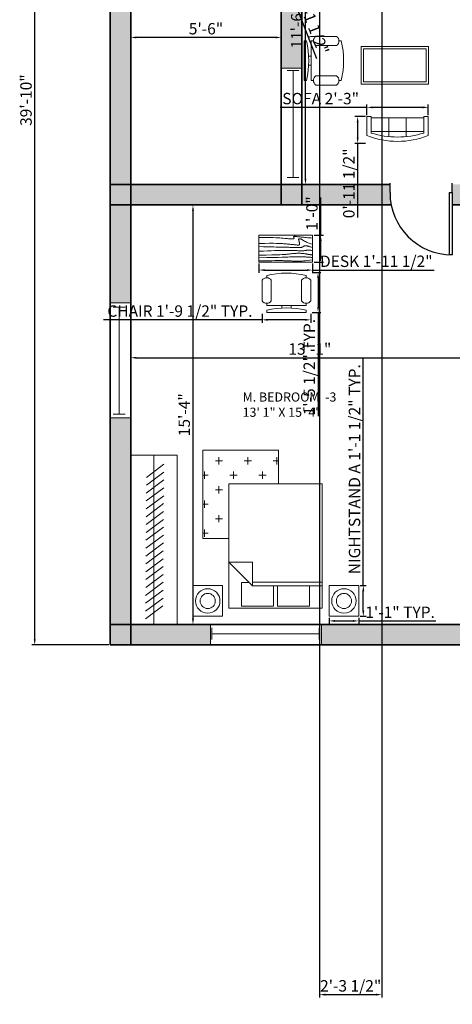
# Model space of a CAD drawing. Units: millimetres. Extents: x 2768 to 4359, y 795 to 1583.
# Tile 1 of 13: x 2772 to 2961, y 854 to 1286. Entities that reach past the tile are written whole.
import ezdxf

# ---------------------------------------------------------------- set-up
doc = ezdxf.new("R2010")
doc.units = ezdxf.units.MM
for name, color, linetype, lineweight in [('A-ANNO-DIMS', 90, 'Continuous', 18), ('A-AREA-IDEN', 190, 'Continuous', 18), ('A-FLOR-CASE', 50, 'Continuous', 18), ('A-FLOR-CASE-PATT', 50, 'Continuous', 13), ('A-FURN-PATT', 50, 'Continuous', 9), ('A-WALL-PATT', 140, 'Continuous', 9), ('doors', 10, 'Continuous', 25), ('furniture', 50, 'Continuous', 18), ('walls', 140, 'Continuous', 35), ('windows', 30, 'Continuous', 18)]:
    doc.layers.add(name, color=color, linetype=linetype, lineweight=lineweight)
doc.styles.get("Standard").update_dxf_attribs({"font": 'arial.ttf'})
doc.dimstyles.new('ISO-25', dxfattribs={"dimtxt": 5, "dimasz": 2.5, "dimexe": 1.25, "dimexo": 0.625, "dimtad": 1, "dimdec": 0, "dimlunit": 3, "dimtxsty": 'Standard', "dimcen": 2.5, "dimadec": 0, "dimazin": 0, "dimtfac": 1, "dimtdec": 0, "dimtmove": 0, "dimatfit": 3, "dimfxl": 1, "dimarcsym": 0})

# ---------------------------------------------------------------- blocks, each defined once
blk = doc.blocks.new('*U2')
for p, q in [((0, 0), (0, -6)), ((40, 0), (40, -6))]:
    blk.add_line(p, q)
blk.add_lwpolyline([(0, 0), (0, 40), (1.75, 40), (1.75, 0)], close=True)
blk.add_arc((0, 0), 40, 0, 90)
blk = doc.blocks.new('*U4')
for p, q in [((0, 4), (0, 0)), ((36, 4), (36, 0)), ((0, 2), (36, 2))]:
    blk.add_line(p, q)
blk = doc.blocks.new('Bed - Queen')
for p, q in [((0, -80.00003), (0, 0)), ((0, 0), (59.99999, 0)), ((59.99999, 0), (59.99999, -80.00003)), ((7.99999, -1.2), (28.79998, -1.2)), ((7.99999, -14.4), (7.99999, -1.2)), ((28.79998, -1.2), (28.79998, -14.4)), ((31.19999, -1.2), (51.99999, -1.2)), ((31.19999, -14.4), (31.19999, -1.2)), ((51.99999, -1.2), (51.99999, -16.4)), ((0, -14.4), (44.8, -14.4)), ((44.8, -16.8), (0, -16.8)), ((59.99999, -29.6), (44.8, -14.4)), ((44.8, -14.4), (44.8, -29.6)), ((51.99999, -16.4), (46.79936, -16.4)), ((44.8, -29.6), (59.99999, -29.6)), ((59.99999, -80.00003), (0, -80.00003))]:
    blk.add_line(p, q)
blk = doc.blocks.new('Chair - Desk')
for p, q in [((-8.5, 0), (-8.5, -1)), ((-8.5, 0), (8.5, 0)), ((8.5, 0), (8.5, -1)), ((-8.5, -3), (-8.5, -4)), ((-8.5, -3), (8.5, -3)), ((-2, -3), (-2, -1.9355)), ((2, -1.9576), (2, -3)), ((8.5, -3), (8.5, -4)), ((-10.5, -5), (-10.5, -14)), ((-6.5, -14), (-6.5, -5)), ((6.5, -5), (6.5, -14)), ((10.5, -14), (10.5, -5)), ((-8.5, -15), (-8.5, -16)), ((8.5, -15), (8.5, -16))]:
    blk.add_line(p, q)
for centre, radius, start, end in [((-8.5, -6.5), 2.5, 36.8699, 143.1301), ((0, 34.625), 36.625, 256.5803, 283.4197), ((8.5, -6.5), 2.5, 36.8699, 143.1301), ((-8.5, -12.5), 2.5, 216.8699, 323.1301), ((0, 19.625), 36.625, 256.5803, 283.4197), ((8.5, -12.5), 2.5, 216.8699, 323.1301)]:
    blk.add_arc(centre, radius, start, end)
blk = doc.blocks.new('Sofa - Roundback 7 ft.')
for p, q in [((-36.000027, -34), (-36.000027, -11.4696)), ((-35.999844, -13.3819), (35.9998, -13.3819)), ((-12.00002, -32.4421), (-12.00003, -6.5971)), ((11.99997, -32.4421), (11.99998, -6.5971)), ((35.99998, -34), (35.99998, -11.4696)), ((-36.000027, -32.4421), (35.99998, -32.4421))]:
    blk.add_line(p, q)
for points in [[(-36.000027, -34), (-42.000027, -34), (-42.000027, -8)], [(41.99998, -8), (41.99998, -34), (35.99998, -34)]]:
    blk.add_lwpolyline(points)
for centre, radius, start, end in [((0, -114.25), 114.25, 68.43141, 111.5686), ((-0.00001, -127.1968), 121.1968, 72.72033, 107.2797)]:
    blk.add_arc(centre, radius, start, end)
blk = doc.blocks.new('Table - Rectangular Woodgrain 60 x 30 in.')
for p, q in [((0, 0), (0, -30)), ((60, 0), (0, 0)), ((60, -30), (60, 0)), ((0, -30), (60, -30))]:
    blk.add_line(p, q)
for points in [[(0, -2.4), (4.8155, -2.418), (9.0302, -2.4688), (12.709, -2.5477), (15.9167, -2.65), (18.7181, -2.7711), (21.1781, -2.9063), (23.3616, -3.0508), (25.3333, -3.2), (27.1477, -3.3495), (28.8172, -3.4958), (30.3437, -3.636), (31.7291, -3.7667), (32.9756, -3.8849), (34.0849, -3.9875), (35.059, -4.0714), (35.9, -4.1334), (36.6114, -4.1711), (37.2041, -4.1854), (37.6906, -4.1779), (38.0833, -4.15), (38.3948, -4.1034), (38.6375, -4.0396), (38.8239, -3.9602), (38.9666, -3.8667), (39.0764, -3.7608), (39.1573, -3.6448), (39.2116, -3.521), (39.2416, -3.3917), (39.2498, -3.2593), (39.2385, -3.1261), (39.21, -2.9944), (39.1666, -2.8667), (39.111, -2.7447), (39.0468, -2.6281), (38.978, -2.5163), (38.9083, -2.4083), (38.8418, -2.3035), (38.7823, -2.201), (38.7337, -2.1001), (38.7, -2), (38.6844, -1.9003), (38.6875, -1.8021), (38.7094, -1.707), (38.75, -1.6167), (38.8094, -1.5326), (38.8875, -1.4563), (38.9844, -1.3893), (39.1, -1.3333), (39.2351, -1.2896), (39.3937, -1.2583), (39.5804, -1.2396), (39.8, -1.2333), (40.057, -1.2396), (40.3562, -1.2583), (40.7023, -1.2896), (41.1, -1.3333), (41.5547, -1.3895), (42.0755, -1.4573), (42.6721, -1.5361), (43.3542, -1.625), (44.1316, -1.7233), (45.014, -1.8302), (46.0114, -1.9449), (47.1333, -2.0667), (48.3862, -2.1947), (49.7625, -2.3281), (51.2513, -2.4663), (52.8416, -2.6083), (54.5226, -2.7535), (56.2833, -2.9011), (58.1127, -3.0501), (60, -3.2)], [(0, -9.2), (6.5759, -9.0858), (11.9385, -9.0365), (16.2527, -9.0418), (19.6833, -9.0917), (22.3952, -9.1759), (24.5531, -9.2844), (26.322, -9.4069), (27.8666, -9.5333), (29.3241, -9.6553), (30.7203, -9.7719), (32.0532, -9.8837), (33.3208, -9.9917), (34.5213, -10.0965), (35.6526, -10.199), (36.7128, -10.2999), (37.7, -10.4), (38.6129, -10.4996), (39.4531, -10.5969), (40.223, -10.6895), (40.925, -10.775), (41.5613, -10.8512), (42.1344, -10.9156), (42.6465, -10.966), (43.1, -11), (43.4976, -11.0158), (43.8437, -11.0136), (44.143, -10.9942), (44.4, -10.9583), (44.6195, -10.9069), (44.8062, -10.8406), (44.9648, -10.7603), (45.1, -10.6667), (45.2155, -10.5598), (45.3114, -10.4365), (45.3871, -10.2929), (45.4416, -10.125), (45.4743, -9.929), (45.4844, -9.7011), (45.4709, -9.4371), (45.4333, -9.1333), (45.3716, -8.7883), (45.2896, -8.4104), (45.1919, -8.0107), (45.0833, -7.6), (44.9685, -7.1893), (44.8521, -6.7896), (44.7388, -6.4117), (44.6333, -6.0667), (44.54, -5.7628), (44.4614, -5.4979), (44.4001, -5.2675), (44.3583, -5.0667), (44.3384, -4.8909), (44.3427, -4.7354), (44.3736, -4.5956), (44.4333, -4.4667), (44.5236, -4.3453), (44.6427, -4.2333), (44.7884, -4.1339), (44.9583, -4.05), (45.1501, -3.9849), (45.3614, -3.9417), (45.59, -3.9234), (45.8333, -3.9333), (46.0915, -3.9749), (46.3734, -4.0531), (46.6906, -4.1736), (47.0542, -4.3417), (47.4756, -4.5629), (47.9661, -4.8427), (48.5372, -5.1866), (49.2, -5.6), (49.9676, -6.0844), (50.8594, -6.625), (51.8965, -7.2031), (53.1, -7.8), (54.491, -8.3969), (56.0906, -8.975), (57.9199, -9.5156), (60, -10)], [(0, -12.8), (5.1847, -12.9322), (9.6213, -13.0323), (13.3963, -13.1059), (16.5958, -13.1583), (19.3063, -13.1952), (21.614, -13.2219), (23.6054, -13.2439), (25.3666, -13.2667), (26.9728, -13.2947), (28.4531, -13.3281), (29.8256, -13.3663), (31.1083, -13.4083), (32.3191, -13.4535), (33.476, -13.501), (34.597, -13.5501), (35.7, -13.6), (36.7984, -13.6497), (37.8875, -13.6979), (38.9578, -13.743), (40, -13.7833), (41.0047, -13.8174), (41.9625, -13.8438), (42.864, -13.8607), (43.7, -13.8667), (44.4631, -13.8604), (45.1552, -13.8417), (45.7801, -13.8104), (46.3416, -13.7667), (46.8439, -13.7104), (47.2906, -13.6417), (47.6858, -13.5604), (48.0333, -13.4667), (48.3375, -13.3608), (48.6042, -13.2448), (48.8396, -13.121), (49.05, -12.9917), (49.2417, -12.8593), (49.4208, -12.7261), (49.5937, -12.5944), (49.7667, -12.4667), (49.9452, -12.3451), (50.1323, -12.2313), (50.3303, -12.1268), (50.5416, -12.0333), (50.7686, -11.9524), (51.0135, -11.8854), (51.2788, -11.8341), (51.5666, -11.8), (51.8785, -11.7843), (52.2116, -11.7865), (52.562, -11.8059), (52.926, -11.8417), (53.2998, -11.8931), (53.6795, -11.9594), (54.0614, -12.0397), (54.4416, -12.1333), (54.8223, -12.2401), (55.2293, -12.3625), (55.6942, -12.5037), (56.2489, -12.6667), (56.9251, -12.8547), (57.7545, -13.0708), (58.7689, -13.3182), (60, -13.6)], [(0, -18), (5.124, -17.7273), (9.6609, -17.5057), (13.6705, -17.3303), (17.2125, -17.1958), (20.3467, -17.0973), (23.1328, -17.0297), (25.6307, -16.9878), (27.9, -16.9667), (29.9928, -16.9617), (31.9302, -16.9703), (33.7254, -16.9907), (35.3917, -17.0208), (36.9423, -17.0588), (38.3906, -17.1026), (39.7499, -17.1503), (41.0333, -17.2), (42.2519, -17.2496), (43.4073, -17.2969), (44.4986, -17.3395), (45.525, -17.375), (46.4858, -17.4012), (47.3802, -17.4156), (48.2074, -17.416), (48.9667, -17.4), (49.6583, -17.3662), (50.2872, -17.3167), (50.8595, -17.2547), (51.3812, -17.1833), (51.8584, -17.1057), (52.2971, -17.025), (52.7034, -16.9443), (53.0833, -16.8667), (53.443, -16.7951), (53.789, -16.7313), (54.128, -16.6768), (54.4666, -16.6334), (54.8115, -16.6024), (55.1693, -16.5854), (55.5465, -16.5841), (55.95, -16.6), (56.3828, -16.6337), (56.8346, -16.6823), (57.2915, -16.7418), (57.7396, -16.8084), (58.165, -16.878), (58.5539, -16.9469), (58.8924, -17.0111), (59.1666, -17.0667), (59.3679, -17.1107), (59.5078, -17.1438), (59.6032, -17.1675), (59.6708, -17.1833), (59.7275, -17.193), (59.7901, -17.1979), (59.8753, -17.1998), (60, -17.2)], [(0, -22.4), (8.0098, -22.2501), (14.4094, -22.1011), (19.4168, -21.9535), (23.25, -21.8083), (26.1269, -21.6663), (28.2656, -21.5281), (29.884, -21.3947), (31.2, -21.2667), (32.3967, -21.1448), (33.5172, -21.0292), (34.5697, -20.9198), (35.5625, -20.8167), (36.5037, -20.7198), (37.4015, -20.6292), (38.2642, -20.5448), (39.1, -20.4667), (39.9164, -20.3951), (40.7187, -20.3313), (41.5117, -20.2768), (42.3, -20.2333), (43.0883, -20.2024), (43.8812, -20.1854), (44.6836, -20.1841), (45.5, -20.2), (46.3328, -20.234), (47.1747, -20.2844), (48.0163, -20.3488), (48.8479, -20.425), (49.66, -20.5106), (50.4429, -20.6031), (51.1872, -20.7004), (51.8833, -20.8), (52.5246, -20.8999), (53.1166, -20.9995), (53.6681, -21.0983), (54.1875, -21.1958), (54.6834, -21.2919), (55.1646, -21.3859), (55.6394, -21.4777), (56.1167, -21.5667), (56.6028, -21.6515), (57.0961, -21.7266), (57.5929, -21.7852), (58.0896, -21.8208), (58.5823, -21.8268), (59.0674, -21.7964), (59.5412, -21.723), (60, -21.6)], [(0, -25.2), (8.6355, -25.0504), (15.7026, -24.9031), (21.4049, -24.7606), (25.9458, -24.625), (29.529, -24.4988), (32.3578, -24.3844), (34.6359, -24.284), (36.5667, -24.2), (38.3213, -24.1341), (39.9417, -24.0854), (41.437, -24.0523), (42.8167, -24.0333), (44.0901, -24.0268), (45.2667, -24.0313), (46.3557, -24.0451), (47.3667, -24.0667), (48.309, -24.0947), (49.1928, -24.1287), (50.0284, -24.168), (50.826, -24.2125), (51.5959, -24.2617), (52.3483, -24.3151), (53.0935, -24.3725), (53.8417, -24.4334), (54.6009, -24.497), (55.3699, -24.561), (56.1454, -24.6226), (56.9239, -24.6792), (57.7021, -24.7279), (58.4764, -24.7662), (59.2435, -24.7911), (60, -24.8)], [(0, -28.8), (5.6867, -28.6681), (10.45, -28.5698), (14.407, -28.5012), (17.675, -28.4584), (20.3711, -28.4374), (22.6125, -28.4344), (24.5164, -28.4455), (26.2, -28.4667), (27.762, -28.4947), (29.2276, -28.5281), (30.6033, -28.5663), (31.8958, -28.6084), (33.1118, -28.6535), (34.2578, -28.7011), (35.3405, -28.7501), (36.3666, -28.8), (37.3443, -28.8497), (38.288, -28.8974), (39.2137, -28.9412), (40.1375, -28.9792), (41.0753, -29.0093), (42.0432, -29.0297), (43.0572, -29.0384), (44.1333, -29.0333), (45.2936, -29.0114), (46.5843, -28.9641), (48.0579, -28.8816), (49.7666, -28.7542), (51.7629, -28.5721), (54.0989, -28.3255), (56.8272, -28.0048), (60, -27.6)]]:
    blk.add_lwpolyline(points)
blk = doc.blocks.new('*D21')
at = {"layer": 'A-ANNO-DIMS', "color": 0, "lineweight": -2, "transparency": 16777216}
for p, q in [((2820.41, 1281.78), (2820.41, 1276.66)), ((2886.41, 1281.78), (2886.41, 1276.66)), ((2883.91, 1277.91), (2822.91, 1277.91))]:
    blk.add_line(p, q, dxfattribs=at)
at = {"layer": 'A-ANNO-DIMS', "color": 0, "transparency": 16777216}
for points in [[(2822.91, 1278.32), (2822.91, 1277.49), (2820.41, 1277.91)], [(2883.91, 1278.32), (2883.91, 1277.49), (2886.41, 1277.91)]]:
    blk.add_solid(points, dxfattribs=at)
at = {"layer": 'Defpoints', "color": 0, "transparency": 16777216}
for p in [(2820.41, 1282.41), (2886.41, 1282.41), (2820.41, 1277.91)]:
    blk.add_point(p, dxfattribs=at)
at = {"layer": 'A-ANNO-DIMS', "color": 0, "transparency": 16777216, "insert": (2853.41, 1281.08), "char_height": 5, "attachment_point": 5}
blk.add_mtext('5\'-6"', dxfattribs=at)
blk = doc.blocks.new('*D22')
at = {"layer": 'A-ANNO-DIMS', "color": 0, "lineweight": -2, "transparency": 16777216}
for p, q in [((2820.41, 1131.43), (2820.41, 1138.66)), ((2822.91, 1137.41), (2974.91, 1137.41)), ((2977.41, 1138.03), (2977.41, 1138.66))]:
    blk.add_line(p, q, dxfattribs=at)
at = {"layer": 'A-ANNO-DIMS', "color": 0, "transparency": 16777216}
for points in [[(2822.91, 1137.82), (2822.91, 1136.99), (2820.41, 1137.41)], [(2974.91, 1137.82), (2974.91, 1136.99), (2977.41, 1137.41)]]:
    blk.add_solid(points, dxfattribs=at)
at = {"layer": 'Defpoints', "color": 0, "transparency": 16777216}
for p in [(2977.41, 1137.41), (2977.41, 1137.41), (2820.41, 1130.8)]:
    blk.add_point(p, dxfattribs=at)
at = {"layer": 'A-ANNO-DIMS', "color": 0, "transparency": 16777216, "insert": (2898.91, 1140.59), "char_height": 5, "attachment_point": 5}
blk.add_mtext('13\'-1"', dxfattribs=at)
blk = doc.blocks.new('*D23')
at = {"layer": 'A-ANNO-DIMS', "color": 0, "lineweight": -2, "transparency": 16777216}
for p, q in [((2844.38, 1204.41), (2848.95, 1204.41)), ((2847.7, 1201.91), (2847.7, 1022.91)), ((2847.38, 1020.41), (2848.95, 1020.41))]:
    blk.add_line(p, q, dxfattribs=at)
at = {"layer": 'A-ANNO-DIMS', "color": 0, "transparency": 16777216}
for points in [[(2847.29, 1201.91), (2848.12, 1201.91), (2847.7, 1204.41)], [(2847.29, 1022.91), (2848.12, 1022.91), (2847.7, 1020.41)]]:
    blk.add_solid(points, dxfattribs=at)
at = {"layer": 'Defpoints', "color": 0, "transparency": 16777216}
for p in [(2843.76, 1204.41), (2846.76, 1020.41), (2847.7, 1020.41)]:
    blk.add_point(p, dxfattribs=at)
at = {"layer": 'A-ANNO-DIMS', "color": 0, "transparency": 16777216, "insert": (2844.52, 1112.41), "char_height": 5, "attachment_point": 5, "rotation": 90}
blk.add_mtext('15\'-4"', dxfattribs=at)
blk = doc.blocks.new('*D31')
at = {"layer": 'A-ANNO-DIMS', "color": 0, "lineweight": -2, "transparency": 16777216}
for p, q in [((2897.01, 1215.91), (2897.01, 1348.91)), ((2897.64, 1351.41), (2898.26, 1351.41)), ((2897.72, 1213.41), (2895.76, 1213.41))]:
    blk.add_line(p, q, dxfattribs=at)
at = {"layer": 'A-ANNO-DIMS', "color": 0, "transparency": 16777216}
for points in [[(2896.59, 1348.91), (2897.43, 1348.91), (2897.01, 1351.41)], [(2896.59, 1215.91), (2897.43, 1215.91), (2897.01, 1213.41)]]:
    blk.add_solid(points, dxfattribs=at)
at = {"layer": 'Defpoints', "color": 0, "transparency": 16777216}
for p in [(2897.01, 1351.41), (2897.01, 1351.41), (2898.34, 1213.41)]:
    blk.add_point(p, dxfattribs=at)
at = {"layer": 'A-ANNO-DIMS', "color": 0, "transparency": 16777216, "insert": (2893.83, 1282.41), "char_height": 5, "attachment_point": 5, "rotation": 90}
blk.add_mtext('11\'-6"', dxfattribs=at)
blk = doc.blocks.new('NIGHTSTAND-RECT-A')
blk.add_lwpolyline([(0, 13.48), (12.92, 13.48), (12.92, 0), (0, 0)], close=True)
for radius in [5.37, 3.33]:
    blk.add_circle((6.46, 6.74), radius)
blk = doc.blocks.new('*D83')
at = {"layer": 'A-ANNO-DIMS', "color": 0, "lineweight": -2, "transparency": 16777216}
for p, q in [((2870.86, 1339.78), (2874.98, 1341.38)), ((2874.71, 1338.6), (2882.05, 1319.7)), ((2880, 1316.23), (2884.12, 1317.83)), ((2882.95, 1317.37), (2901.88, 1268.61))]:
    blk.add_line(p, q, dxfattribs=at)
at = {"layer": 'A-ANNO-DIMS', "color": 0, "transparency": 16777216}
for points in [[(2875.1, 1338.75), (2874.33, 1338.45), (2873.81, 1340.93)], [(2882.44, 1319.85), (2881.66, 1319.55), (2882.95, 1317.37)]]:
    blk.add_solid(points, dxfattribs=at)
at = {"layer": 'Defpoints', "color": 0, "transparency": 16777216}
for p in [(2870.28, 1339.56), (2882.95, 1317.37), (2879.42, 1316)]:
    blk.add_point(p, dxfattribs=at)
at = {"layer": 'A-ANNO-DIMS', "color": 0, "transparency": 16777216, "insert": (2895.86, 1292.99), "char_height": 5, "attachment_point": 5, "rotation": 291.2165}
blk.add_mtext('CHAIR 2\'-1 1/2"', dxfattribs=at)
blk = doc.blocks.new('*D85')
at = {"layer": 'A-ANNO-DIMS', "color": 0, "lineweight": -2, "transparency": 16777216}
for p, q in [((2877.97, 1154.03), (2808.48, 1154.03)), ((2877.97, 1156.61), (2877.97, 1152.78)), ((2896.83, 1154.03), (2880.47, 1154.03)), ((2899.33, 1156.61), (2899.33, 1152.78))]:
    blk.add_line(p, q, dxfattribs=at)
at = {"layer": 'A-ANNO-DIMS', "color": 0, "transparency": 16777216}
for points in [[(2880.47, 1154.45), (2880.47, 1153.62), (2877.97, 1154.03)], [(2896.83, 1154.45), (2896.83, 1153.62), (2899.33, 1154.03)]]:
    blk.add_solid(points, dxfattribs=at)
at = {"layer": 'Defpoints', "color": 0, "transparency": 16777216}
for p in [(2877.97, 1157.23), (2877.97, 1154.03), (2899.33, 1157.23)]:
    blk.add_point(p, dxfattribs=at)
at = {"layer": 'A-ANNO-DIMS', "color": 0, "transparency": 16777216, "insert": (2841.98, 1157.24), "char_height": 5, "attachment_point": 5}
blk.add_mtext('CHAIR 1\'-9 1/2" TYP.', dxfattribs=at)
blk = doc.blocks.new('*D86')
at = {"layer": 'A-ANNO-DIMS', "color": 0, "lineweight": -2, "transparency": 16777216}
for p, q in [((2899.95, 1174.86), (2903.78, 1174.86)), ((2902.53, 1172.36), (2902.53, 1159.73)), ((2899.95, 1157.23), (2903.78, 1157.23)), ((2902.53, 1157.23), (2902.53, 1111.83))]:
    blk.add_line(p, q, dxfattribs=at)
at = {"layer": 'A-ANNO-DIMS', "color": 0, "transparency": 16777216}
for points in [[(2902.11, 1172.36), (2902.95, 1172.36), (2902.53, 1174.86)], [(2902.11, 1159.73), (2902.95, 1159.73), (2902.53, 1157.23)]]:
    blk.add_solid(points, dxfattribs=at)
at = {"layer": 'Defpoints', "color": 0, "transparency": 16777216}
for p in [(2899.33, 1174.86), (2899.33, 1157.23), (2902.53, 1157.23)]:
    blk.add_point(p, dxfattribs=at)
at = {"layer": 'A-ANNO-DIMS', "color": 0, "transparency": 16777216, "insert": (2899.32, 1133.28), "char_height": 5, "attachment_point": 5, "rotation": 90}
blk.add_mtext('1\'-5 1/2" TYP.', dxfattribs=at)
blk = doc.blocks.new('*D101')
at = {"layer": 'A-ANNO-DIMS', "color": 0, "lineweight": -2, "transparency": 16777216}
for p, q in [((2923.9, 1243.81), (2923.9, 1248.47)), ((2950.8, 1243.81), (2950.8, 1248.47)), ((2923.9, 1247.22), (2885.92, 1247.22)), ((2948.3, 1247.22), (2926.4, 1247.22))]:
    blk.add_line(p, q, dxfattribs=at)
at = {"layer": 'A-ANNO-DIMS', "color": 0, "transparency": 16777216}
for points in [[(2926.4, 1247.64), (2926.4, 1246.81), (2923.9, 1247.22)], [(2948.3, 1247.64), (2948.3, 1246.81), (2950.8, 1247.22)]]:
    blk.add_solid(points, dxfattribs=at)
at = {"layer": 'Defpoints', "color": 0, "transparency": 16777216}
for p in [(2923.9, 1247.22), (2923.9, 1243.19), (2950.8, 1243.19)]:
    blk.add_point(p, dxfattribs=at)
at = {"layer": 'A-ANNO-DIMS', "color": 0, "transparency": 16777216, "insert": (2903.66, 1250.44), "char_height": 5, "attachment_point": 5}
blk.add_mtext('SOFA 2\'-3"', dxfattribs=at)
blk = doc.blocks.new('*D102')
at = {"layer": 'A-ANNO-DIMS', "color": 0, "lineweight": -2, "transparency": 16777216}
for p, q in [((2923.28, 1243.19), (2918.62, 1243.19)), ((2919.87, 1240.69), (2919.87, 1233.95)), ((2923.28, 1231.45), (2918.62, 1231.45)), ((2919.87, 1231.45), (2919.87, 1198.87))]:
    blk.add_line(p, q, dxfattribs=at)
at = {"layer": 'A-ANNO-DIMS', "color": 0, "transparency": 16777216}
for points in [[(2919.45, 1240.69), (2920.28, 1240.69), (2919.87, 1243.19)], [(2919.45, 1233.95), (2920.28, 1233.95), (2919.87, 1231.45)]]:
    blk.add_solid(points, dxfattribs=at)
at = {"layer": 'Defpoints', "color": 0, "transparency": 16777216}
for p in [(2923.9, 1243.19), (2919.87, 1231.45), (2923.9, 1231.45)]:
    blk.add_point(p, dxfattribs=at)
at = {"layer": 'A-ANNO-DIMS', "color": 0, "transparency": 16777216, "insert": (2916.66, 1213.91), "char_height": 5, "attachment_point": 5, "rotation": 90}
blk.add_mtext('0\'-11 1/2"', dxfattribs=at)
blk = doc.blocks.new('*D113')
at = {"layer": 'A-ANNO-DIMS', "color": 0, "lineweight": -2, "transparency": 16777216}
for p, q in [((2876.62, 1178.77), (2876.62, 1174.61)), ((2879.12, 1175.86), (2897.64, 1175.86)), ((2900.14, 1178.77), (2900.14, 1174.61)), ((2900.14, 1175.86), (2953.43, 1175.86))]:
    blk.add_line(p, q, dxfattribs=at)
at = {"layer": 'A-ANNO-DIMS', "color": 0, "transparency": 16777216}
for points in [[(2879.12, 1176.28), (2879.12, 1175.45), (2876.62, 1175.86)], [(2897.64, 1176.28), (2897.64, 1175.45), (2900.14, 1175.86)]]:
    blk.add_solid(points, dxfattribs=at)
at = {"layer": 'Defpoints', "color": 0, "transparency": 16777216}
for p in [(2876.62, 1179.39), (2900.14, 1179.39), (2900.14, 1175.86)]:
    blk.add_point(p, dxfattribs=at)
at = {"layer": 'A-ANNO-DIMS', "color": 0, "transparency": 16777216, "insert": (2928.04, 1179.07), "char_height": 5, "attachment_point": 5}
blk.add_mtext('DESK 1\'-11 1/2"', dxfattribs=at)
blk = doc.blocks.new('*D114')
at = {"layer": 'A-ANNO-DIMS', "color": 0, "lineweight": -2, "transparency": 16777216}
for p, q in [((2903.67, 1191.15), (2903.67, 1207.72)), ((2900.77, 1191.15), (2904.92, 1191.15)), ((2903.67, 1181.89), (2903.67, 1188.65)), ((2900.77, 1179.39), (2904.92, 1179.39))]:
    blk.add_line(p, q, dxfattribs=at)
at = {"layer": 'A-ANNO-DIMS', "color": 0, "transparency": 16777216}
for points in [[(2903.25, 1188.65), (2904.09, 1188.65), (2903.67, 1191.15)], [(2903.25, 1181.89), (2904.09, 1181.89), (2903.67, 1179.39)]]:
    blk.add_solid(points, dxfattribs=at)
at = {"layer": 'Defpoints', "color": 0, "transparency": 16777216}
for p in [(2900.14, 1191.15), (2903.67, 1191.15), (2900.14, 1179.39)]:
    blk.add_point(p, dxfattribs=at)
at = {"layer": 'A-ANNO-DIMS', "color": 0, "transparency": 16777216, "insert": (2900.49, 1200.69), "char_height": 5, "attachment_point": 5, "rotation": 90}
blk.add_mtext('1\'-0"', dxfattribs=at)
blk = doc.blocks.new('*D117')
at = {"layer": 'A-ANNO-DIMS', "color": 0, "lineweight": -2, "transparency": 16777216}
for p, q in [((2922.35, 1037.47), (2922.35, 1137.05)), ((2920.95, 1037.47), (2923.6, 1037.47)), ((2922.35, 1026.48), (2922.35, 1034.97)), ((2920.95, 1023.98), (2923.6, 1023.98))]:
    blk.add_line(p, q, dxfattribs=at)
at = {"layer": 'A-ANNO-DIMS', "color": 0, "transparency": 16777216}
for points in [[(2921.93, 1034.97), (2922.77, 1034.97), (2922.35, 1037.47)], [(2921.93, 1026.48), (2922.77, 1026.48), (2922.35, 1023.98)]]:
    blk.add_solid(points, dxfattribs=at)
at = {"layer": 'Defpoints', "color": 0, "transparency": 16777216}
for p in [(2920.33, 1037.47), (2922.35, 1037.47), (2920.33, 1023.98)]:
    blk.add_point(p, dxfattribs=at)
at = {"layer": 'A-ANNO-DIMS', "color": 0, "transparency": 16777216, "insert": (2919.14, 1088.51), "char_height": 5, "attachment_point": 5, "rotation": 90}
blk.add_mtext('NIGHTSTAND A 1\'-1 1/2" TYP.', dxfattribs=at)
blk = doc.blocks.new('*D118')
at = {"layer": 'A-ANNO-DIMS', "color": 0, "lineweight": -2, "transparency": 16777216}
for p, q in [((2907.41, 1023.36), (2907.41, 1020.71)), ((2909.91, 1021.96), (2917.83, 1021.96)), ((2920.33, 1023.36), (2920.33, 1020.71)), ((2920.33, 1021.96), (2954.08, 1021.96))]:
    blk.add_line(p, q, dxfattribs=at)
at = {"layer": 'A-ANNO-DIMS', "color": 0, "transparency": 16777216}
for points in [[(2909.91, 1022.38), (2909.91, 1021.54), (2907.41, 1021.96)], [(2917.83, 1022.38), (2917.83, 1021.54), (2920.33, 1021.96)]]:
    blk.add_solid(points, dxfattribs=at)
at = {"layer": 'Defpoints', "color": 0, "transparency": 16777216}
for p in [(2907.41, 1023.98), (2920.33, 1023.98), (2920.33, 1021.96)]:
    blk.add_point(p, dxfattribs=at)
at = {"layer": 'A-ANNO-DIMS', "color": 0, "transparency": 16777216, "insert": (2938.46, 1025.1), "char_height": 5, "attachment_point": 5}
blk.add_mtext('1\'-1" TYP.', dxfattribs=at)
blk = doc.blocks.new('*D127')
at = {"layer": 'A-ANNO-DIMS', "color": 0, "lineweight": -2, "transparency": 16777216}
for p, q in [((2810.78, 1489.41), (2777.11, 1489.41)), ((2778.36, 1013.91), (2778.36, 1486.91)), ((2810.78, 1011.41), (2777.11, 1011.41))]:
    blk.add_line(p, q, dxfattribs=at)
at = {"layer": 'A-ANNO-DIMS', "color": 0, "transparency": 16777216}
for points in [[(2777.94, 1486.91), (2778.77, 1486.91), (2778.36, 1489.41)], [(2777.94, 1013.91), (2778.77, 1013.91), (2778.36, 1011.41)]]:
    blk.add_solid(points, dxfattribs=at)
at = {"layer": 'Defpoints', "color": 0, "transparency": 16777216}
for p in [(2778.36, 1489.41), (2811.41, 1489.41), (2811.41, 1011.41)]:
    blk.add_point(p, dxfattribs=at)
at = {"layer": 'A-ANNO-DIMS', "color": 0, "transparency": 16777216, "insert": (2775.18, 1250.41), "char_height": 5, "attachment_point": 5, "rotation": 90}
blk.add_mtext('39\'-10"', dxfattribs=at)
blk = doc.blocks.new('*D133')
at = {"layer": 'A-ANNO-DIMS', "color": 0, "lineweight": -2, "transparency": 16777216}
for p, q in [((2903.16, 1350.78), (2903.16, 856.79)), ((2930.46, 1350.78), (2930.46, 856.79)), ((2905.66, 858.04), (2927.96, 858.04))]:
    blk.add_line(p, q, dxfattribs=at)
at = {"layer": 'A-ANNO-DIMS', "color": 0, "transparency": 16777216}
for points in [[(2905.66, 858.46), (2905.66, 857.63), (2903.16, 858.04)], [(2927.96, 858.46), (2927.96, 857.63), (2930.46, 858.04)]]:
    blk.add_solid(points, dxfattribs=at)
at = {"layer": 'Defpoints', "color": 0, "transparency": 16777216}
for p in [(2903.16, 1351.41), (2930.46, 1351.41), (2930.46, 858.04)]:
    blk.add_point(p, dxfattribs=at)
at = {"layer": 'A-ANNO-DIMS', "color": 0, "transparency": 16777216, "insert": (2916.81, 861.25), "char_height": 5, "attachment_point": 5}
blk.add_mtext('2\'-3 1/2"', dxfattribs=at)

msp = doc.modelspace()

# ---------------------------------------------------------------- hatches: boundary and pattern name
at = {"layer": 'A-FLOR-CASE-PATT'}
h = msp.add_hatch(dxfattribs=at)
h.set_pattern_fill('ANSI31', color=256, scale=0.865728, angle=-8.151, style=0)
h.paths.add_polyline_path([(2834.54, 1027.06), (2826.88, 1021.32), (2827.3, 1086.9), (2834.96, 1092.64)])
at = {"layer": 'A-FURN-PATT'}
h = msp.add_hatch(dxfattribs=at)
h.set_pattern_fill('CROSS', color=256)
h.paths.add_polyline_path([(2885.16, 1096.89), (2852.08, 1096.89), (2852.08, 1058.14), (2863.47, 1058.14), (2863.47, 1082.02), (2885.16, 1082.02)])
at = {"layer": 'A-WALL-PATT'}
h = msp.add_hatch(color=256, dxfattribs=at)
h.dxf.hatch_style = 1
h.paths.add_polyline_path([(2820.41, 1480.41), (2811.41, 1480.41), (2811.41, 1360.41), (2820.41, 1360.41)])
h.paths.add_polyline_path([(2820.41, 1489.41), (2811.41, 1489.41), (2811.41, 1480.41), (2820.41, 1480.41)])
h.paths.add_polyline_path([(2845.83, 1489.41), (2820.41, 1489.41), (2820.41, 1480.41), (2845.83, 1480.41)])
h.paths.add_polyline_path([(2940.41, 1489.41), (2894.95, 1489.41), (2894.95, 1480.41), (2940.41, 1480.41)])
h.paths.add_polyline_path([(2949.41, 1489.41), (2940.41, 1489.41), (2940.41, 1480.41), (2949.41, 1480.41)])
h.paths.add_polyline_path([(2949.41, 1480.41), (2940.41, 1480.41), (2940.41, 1433.68), (2943.15, 1433.68), (2949.41, 1433.68)])
h.paths.add_polyline_path([(2964.2, 1489.41), (2949.41, 1489.41), (2949.41, 1480.41), (2964.2, 1480.41)])
h.paths.add_polyline_path([(3018.41, 1489.41), (3009.41, 1489.41), (3009.41, 1480.41), (3018.41, 1480.41)])
h.paths.add_polyline_path([(3009.41, 1489.41), (2990.92, 1489.41), (2990.92, 1480.41), (3009.41, 1480.41)])
h.paths.add_polyline_path([(3018.41, 1480.41), (3009.41, 1480.41), (3009.41, 1384.41), (3018.41, 1384.41)])
h.paths.add_polyline_path([(3009.41, 1384.41), (2949.41, 1384.41), (2949.41, 1375.41), (3009.41, 1375.41)])
h.paths.add_polyline_path([(3018.41, 1384.41), (3009.41, 1384.41), (3009.41, 1375.41), (3018.41, 1375.41)])
h.paths.add_polyline_path([(2949.41, 1384.41), (2940.41, 1384.41), (2940.41, 1375.41), (2949.41, 1375.41)])
h.paths.add_polyline_path([(2949.41, 1413.64, -0.075856), (2943.15, 1412.69), (2940.41, 1412.69), (2940.41, 1384.41), (2949.41, 1384.41)])
h.paths.add_polyline_path([(2949.41, 1375.41), (2940.41, 1375.41), (2940.41, 1360.41), (2949.41, 1360.41)])
h.paths.add_polyline_path([(2949.41, 1360.41), (2940.41, 1360.41), (2940.41, 1351.41), (2949.41, 1351.41)])
h.paths.add_polyline_path([(2940.41, 1360.41), (2929.82, 1360.41, -0.054277), (2930.46, 1354.53), (2930.46, 1351.41), (2940.41, 1351.41)])
h.paths.add_polyline_path([(2903.16, 1354.53), (2903.16, 1360.41), (2895.41, 1360.41), (2895.41, 1351.41), (2903.16, 1351.41)])
h.paths.add_polyline_path([(2886.41, 1360.41), (2820.41, 1360.41), (2820.41, 1351.41), (2886.41, 1351.41)])
h.paths.add_polyline_path([(2895.41, 1360.41), (2886.41, 1360.41), (2886.41, 1351.41), (2895.41, 1351.41)])
h.paths.add_polyline_path([(2820.41, 1360.41), (2811.41, 1360.41), (2811.41, 1351.41), (2820.41, 1351.41)])
h.paths.add_polyline_path([(2820.41, 1351.41), (2811.41, 1351.41), (2811.41, 1213.41), (2820.41, 1213.41)])
h.paths.add_polyline_path([(2886.41, 1213.41), (2820.41, 1213.41), (2820.41, 1204.41), (2886.41, 1204.41)])
h.paths.add_polyline_path([(2820.41, 1213.41), (2811.41, 1213.41), (2811.41, 1204.41), (2820.41, 1204.41)])
h.paths.add_polyline_path([(2895.41, 1302), (2886.41, 1302), (2886.41, 1264.47), (2895.41, 1264.47)])
h.paths.add_polyline_path([(2934.05, 1209.82), (2934.05, 1213.41), (2895.41, 1213.41), (2895.41, 1204.41), (2934.59, 1204.41, -0.049949)])
h.paths.add_polyline_path([(2895.41, 1213.41), (2886.41, 1213.41), (2886.41, 1204.41), (2895.41, 1204.41)])
h.paths.add_polyline_path([(3078.41, 1384.41), (3018.41, 1384.41), (3018.41, 1375.41), (3078.41, 1375.41)])
h.paths.add_polyline_path([(3087.41, 1433.68), (3084.62, 1433.68), (3078.41, 1433.68), (3078.41, 1384.41), (3087.41, 1384.41)])
h.paths.add_polyline_path([(3087.41, 1384.41), (3078.41, 1384.41), (3078.41, 1375.41), (3087.41, 1375.41)])
h.paths.add_polyline_path([(3087.41, 1375.41), (3078.41, 1375.41), (3078.41, 1360.41), (3087.41, 1360.41)])
h.paths.add_polyline_path([(3087.41, 1360.41), (3078.41, 1360.41), (3078.41, 1351.41), (3087.41, 1351.41)])
h.paths.add_polyline_path([(3093.5, 1360.41), (3087.41, 1360.41), (3087.41, 1351.41), (3093.5, 1351.41), (3093.5, 1353.18)])
h.paths.add_polyline_path([(3207.41, 1360.41), (3119.82, 1360.41, -0.067042), (3120.8, 1353.18), (3120.8, 1351.41), (3207.41, 1351.41)])
h.paths.add_polyline_path([(3216.41, 1480.41), (3207.41, 1480.41), (3207.41, 1360.41), (3216.41, 1360.41)])
h.paths.add_polyline_path([(3216.41, 1360.41), (3207.41, 1360.41), (3207.41, 1351.41), (3216.41, 1351.41)])
h.paths.add_polyline_path([(3216.41, 1489.41), (3207.41, 1489.41), (3207.41, 1480.41), (3216.41, 1480.41)])
h.paths.add_polyline_path([(3207.41, 1489.41), (3167.11, 1489.41), (3167.11, 1480.41), (3207.41, 1480.41)])
h.paths.add_polyline_path([(3118.27, 1489.41), (3087.41, 1489.41), (3087.41, 1480.41), (3118.27, 1480.41)])
h.paths.add_polyline_path([(3087.41, 1489.41), (3078.41, 1489.41), (3078.41, 1480.41), (3087.41, 1480.41)])
h.paths.add_polyline_path([(3087.41, 1480.41), (3078.41, 1480.41), (3078.41, 1453.72, -0.07525), (3084.62, 1454.66), (3087.41, 1454.66)])
h.paths.add_polyline_path([(3078.41, 1489.41), (3058.65, 1489.41), (3058.65, 1480.41), (3078.41, 1480.41)])
h.paths.add_polyline_path([(3031.86, 1489.41), (3018.41, 1489.41), (3018.41, 1480.41), (3031.86, 1480.41)])
h.paths.add_polyline_path([(3458.41, 1489.41), (3216.41, 1489.41), (3216.41, 1480.41), (3458.41, 1480.41)])
h.paths.add_polyline_path([(3467.41, 1489.41), (3458.41, 1489.41), (3458.41, 1480.41), (3467.41, 1480.41)])
h.paths.add_polyline_path([(3467.41, 1480.41), (3458.41, 1480.41), (3458.41, 1020.41), (3467.41, 1020.41)])
h.paths.add_polyline_path([(3458.41, 1020.41), (3216.41, 1020.41), (3216.41, 1011.41), (3458.41, 1011.41)])
h.paths.add_polyline_path([(3467.41, 1020.41), (3458.41, 1020.41), (3458.41, 1011.41), (3467.41, 1011.41)])
h.paths.add_polyline_path([(3216.41, 1080.41), (3207.41, 1080.41), (3207.41, 1020.41), (3216.41, 1020.41)])
h.paths.add_polyline_path([(3216.41, 1020.41), (3207.41, 1020.41), (3207.41, 1011.41), (3216.41, 1011.41)])
h.paths.add_polyline_path([(3207.41, 1020.41), (3151.59, 1020.41), (3151.59, 1011.41), (3207.41, 1011.41)])
h.paths.add_polyline_path([(3216.41, 1185.41), (3207.41, 1185.41), (3207.41, 1089.41), (3216.41, 1089.41)])
h.paths.add_polyline_path([(3216.41, 1089.41), (3207.41, 1089.41), (3207.41, 1080.41), (3216.41, 1080.41)])
h.paths.add_polyline_path([(3207.41, 1089.41), (3097.07, 1089.41), (3097.07, 1087.42), (3097.07, 1080.41), (3207.41, 1080.41)])
h.paths.add_polyline_path([(3216.41, 1194.41), (3207.41, 1194.41), (3207.41, 1185.41), (3216.41, 1185.41)])
h.paths.add_polyline_path([(3207.41, 1194.41), (3055.41, 1194.41), (3055.41, 1185.41), (3207.41, 1185.41)])
h.paths.add_polyline_path([(3055.41, 1194.41), (3046.41, 1194.41), (3046.41, 1185.41), (3055.41, 1185.41)])
h.paths.add_polyline_path([(3055.41, 1128.41), (3046.41, 1128.41), (3046.41, 1020.41), (3055.41, 1020.41)])
h.paths.add_polyline_path([(3055.41, 1020.41), (3046.41, 1020.41), (3046.41, 1011.41), (3055.41, 1011.41)])
h.paths.add_polyline_path([(3102.66, 1020.41), (3055.41, 1020.41), (3055.41, 1011.41), (3102.66, 1011.41)])
h.paths.add_polyline_path([(3055.41, 1137.41), (3046.41, 1137.41), (3046.41, 1128.41), (3055.41, 1128.41)])
h.paths.add_polyline_path([(3046.41, 1137.41), (2986.41, 1137.41), (2986.41, 1128.41), (3046.41, 1128.41)])
h.paths.add_polyline_path([(2986.41, 1204.41), (2977.41, 1204.41), (2977.41, 1137.41), (2986.41, 1137.41)])
h.paths.add_polyline_path([(2986.41, 1213.41), (2977.41, 1213.41), (2977.41, 1204.41), (2986.41, 1204.41)])
h.paths.add_polyline_path([(2977.41, 1213.41), (2961.35, 1213.41), (2961.35, 1209.82), (2961.35, 1204.41), (2977.41, 1204.41)])
h.paths.add_polyline_path([(2986.41, 1137.41), (2977.41, 1137.41), (2977.41, 1128.41), (2986.41, 1128.41)])
h.paths.add_polyline_path([(2986.41, 1128.41), (2977.41, 1128.41), (2977.41, 1073.04), (2980.14, 1073.04), (2986.41, 1073.04)])
h.paths.add_polyline_path([(2986.41, 1053, -0.075909), (2980.14, 1052.05), (2977.41, 1052.05), (2977.41, 1020.41), (2986.41, 1020.41)])
h.paths.add_polyline_path([(2986.41, 1020.41), (2977.41, 1020.41), (2977.41, 1011.41), (2986.41, 1011.41)])
h.paths.add_polyline_path([(2977.41, 1020.41), (2903.99, 1020.41), (2903.99, 1011.41), (2977.41, 1011.41)])
h.paths.add_polyline_path([(2820.41, 1111.04), (2811.41, 1111.04), (2811.41, 1020.41), (2820.41, 1020.41)])
h.paths.add_polyline_path([(2820.41, 1020.41), (2811.41, 1020.41), (2811.41, 1011.41), (2820.41, 1011.41)])
h.paths.add_polyline_path([(2855.32, 1020.41), (2820.41, 1020.41), (2820.41, 1011.41), (2855.32, 1011.41)])
h.paths.add_polyline_path([(2820.41, 1204.41), (2811.41, 1204.41), (2811.41, 1161.45), (2820.41, 1161.45)])
edge = h.paths.add_edge_path()
edge.add_arc((3211.84, 1295.2), 27.3, 86.9636, 99.352)
edge.add_line((3207.41, 1322.13), (3207.41, 1351.41))
edge.add_line((3207.41, 1351.41), (3216.41, 1351.41))
edge.add_line((3216.41, 1351.41), (3216.41, 1322.29))
edge.add_line((3216.41, 1322.29), (3213.29, 1322.46))

# ---------------------------------------------------------------- linework, layer by layer
at = {"layer": 'A-FLOR-CASE'}
msp.add_line((2830.58, 1094.68), (2830.58, 1020.41), dxfattribs=at)
msp.add_lwpolyline([(2820.41, 1020.41), (2840.74, 1020.41), (2840.74, 1094.68), (2820.41, 1094.68)], close=True, dxfattribs=at)
at = {"layer": 'furniture'}
for points in [[(2921.41, 1273.97), (2950.95, 1273.97), (2950.95, 1257.39), (2921.41, 1257.39)], [(2922.41, 1272.97), (2949.95, 1272.97), (2949.95, 1258.39), (2922.41, 1258.39)]]:
    msp.add_lwpolyline(points, close=True, dxfattribs=at)
msp.add_lwpolyline([(2863.47, 1058.14), (2852.08, 1058.14), (2852.08, 1096.89), (2885.16, 1096.89), (2885.16, 1082.02)], dxfattribs=at)
at = {"layer": 'walls'}
for p, q in [((2811.41, 1489.41), (2811.41, 1011.41)), ((2886.41, 1360.41), (2886.41, 1204.41)), ((2895.41, 1360.41), (2895.41, 1204.41)), ((2820.41, 1351.41), (2820.41, 1204.41)), ((2811.41, 1213.41), (2934.05, 1213.41)), ((2811.41, 1204.41), (2934.59, 1204.41)), ((2820.41, 1204.41), (2820.41, 1011.41)), ((2961.35, 1204.41), (2986.41, 1204.41)), ((2811.41, 1020.41), (3055.41, 1020.41)), ((2811.41, 1011.41), (3055.41, 1011.41))]:
    msp.add_line(p, q, dxfattribs=at)
at = {"layer": 'windows'}
for p, q in [((2895.41, 1264.47), (2886.41, 1264.47)), ((2820.41, 1161.45), (2811.41, 1161.45)), ((2820.41, 1111.04), (2811.41, 1111.04)), ((2855.32, 1020.41), (2855.32, 1011.41)), ((2903.99, 1011.41), (2903.99, 1020.41))]:
    msp.add_line(p, q, dxfattribs=at)

# ---------------------------------------------------------------- block references
at = {"layer": 'doors', "xscale": 0.6824775533392957, "yscale": 0.6824775533392957, "zscale": 0.6824775533392957, "rotation": 180}
msp.add_blockref('*U2', (2961.35, 1209.82), dxfattribs=at)
at = {"layer": 'furniture'}
for name, p, xscale, yscale, zscale, rotation in [('Chair - Desk', (2896.43, 1267.71), 1.016793948962143, 1.016793948962143, 1.016793948962143, 90), ('Sofa - Roundback 7 ft.', (2937.35, 1232.3), 0.3202410777606914, 0.3202410777606914, 0.3202410777606914, 180), ('Chair - Desk', (2888.65, 1157.23), 1.016793948962143, 1.016793948962143, 1.016793948962143, 180), ('Bed - Queen', (2904.28, 1027.61), 0.6802112050549222, 0.6802112050549222, 0.6802112050549222, 180)]:
    msp.add_blockref(name, p, dxfattribs=dict(at, xscale=xscale, yscale=yscale, zscale=zscale, rotation=rotation))
at = {"layer": 'furniture', "xscale": 0.3920057089081217, "yscale": 0.3920057089081217, "zscale": 0.3920057089081217}
msp.add_blockref('Table - Rectangular Woodgrain 60 x 30 in.', (2876.62, 1191.15), dxfattribs=at)
at = {"layer": 'furniture'}
for p in [(2847.7, 1023.98), (2907.41, 1023.98)]:
    msp.add_blockref('NIGHTSTAND-RECT-A', p, dxfattribs=at)
at = {"layer": 'windows', "xscale": 1.304585616368386, "yscale": 1.304585616368386, "zscale": 1.304585616368386, "rotation": 90}
for p in [(2894.16, 1216.49), (2817.93, 1112.61)]:
    msp.add_blockref('*U4', p, dxfattribs=at)
at = {"layer": 'windows', "xscale": 1.304585616368386, "yscale": 1.304585616368386, "zscale": 1.304585616368386}
msp.add_blockref('*U4', (2855.99, 1013.75), dxfattribs=at)

# ---------------------------------------------------------------- texts
at = {"layer": 'A-AREA-IDEN', "insert": (2869.46, 1122.18), "char_height": 4, "attachment_point": 1}
msp.add_mtext_dynamic_manual_height_columns('M. BEDROOM  -3 \\P13\' 1" X 15\' 4"', width=87.9766, gutter_width=12.5, heights=[0], dxfattribs=at)

# ---------------------------------------------------------------- dimensions: what is measured, and where the dimension line sits
at = {"layer": 'A-ANNO-DIMS'}
for base, p1, p2, angle, override, picture, middle in [((2778.36, 1489.41), (2811.41, 1011.41), (2811.41, 1489.41), 90, {"dimdec": 1, "dimlfac": 1, "dimrnd": 0, "dimzin": 1, "dimdsep": 46, "dimlunit": 4, "dimfrac": 2}, '*D127', (2775.18, 1250.41)), ((2897.01, 1351.41), (2898.34, 1213.41), (2897.01, 1351.41), 90, {"dimclrd": 0, "dimclre": 0, "dimclrt": 0}, '*D31', (2893.83, 1282.41)), ((2919.87, 1231.45), (2923.9, 1243.19), (2923.9, 1231.45), 270, {"dimdec": 1, "dimlfac": 1, "dimrnd": 0, "dimzin": 1, "dimdsep": 46, "dimlunit": 4, "dimfrac": 2}, '*D102', (2916.66, 1213.91)), ((2903.67, 1191.15), (2900.14, 1179.39), (2900.14, 1191.15), 90, {"dimdec": 1, "dimlfac": 1, "dimrnd": 0, "dimzin": 1, "dimdsep": 46, "dimlunit": 4, "dimfrac": 2}, '*D114', (2900.49, 1200.69)), ((2847.7, 1020.41), (2843.76, 1204.41), (2846.76, 1020.41), 90, {"dimclrd": 0, "dimclre": 0, "dimclrt": 0}, '*D23', (2844.52, 1112.41))]:
    dim = msp.add_linear_dim(base=base, p1=p1, p2=p2, angle=angle, dimstyle='ISO-25', override=override, dxfattribs=at)
    dim.commit()
    dim.dimension.update_dxf_attribs({"geometry": picture, "text_midpoint": middle})
for base, p1, p2, override, picture, middle in [((2930.46, 858.04), (2903.16, 1351.41), (2930.46, 1351.41), {"dimdec": 1, "dimlfac": 1, "dimrnd": 0, "dimzin": 1, "dimdsep": 46, "dimlunit": 4, "dimfrac": 2}, '*D133', (2916.81, 861.25)), ((2820.41, 1277.91), (2886.41, 1282.41), (2820.41, 1282.41), {"dimclrd": 0, "dimclre": 0, "dimclrt": 0}, '*D21', (2853.41, 1281.08)), ((2977.41, 1137.41), (2820.41, 1130.8), (2977.41, 1137.41), {"dimclrd": 0, "dimclre": 0, "dimclrt": 0}, '*D22', (2898.91, 1140.59))]:
    dim = msp.add_linear_dim(base=base, p1=p1, p2=p2, dimstyle='ISO-25', override=override, dxfattribs=at)
    dim.commit()
    dim.dimension.update_dxf_attribs({"geometry": picture, "text_midpoint": middle})
for base, p1, p2, angle, text, picture, middle in [((2882.95, 1317.37), (2870.28, 1339.56), (2879.42, 1316), 291.2165, 'CHAIR <>', '*D83', (2895.86, 1292.99)), ((2923.9, 1247.22), (2950.8, 1243.19), (2923.9, 1243.19), 180, 'SOFA <>', '*D101', (2903.66, 1250.44)), ((2902.53, 1157.23), (2899.33, 1174.86), (2899.33, 1157.23), 270, '<> TYP.', '*D86', (2899.32, 1133.28)), ((2877.97, 1154.03), (2899.33, 1157.23), (2877.97, 1157.23), 180, 'CHAIR <> TYP.', '*D85', (2841.98, 1157.24)), ((2922.35, 1037.47), (2920.33, 1023.98), (2920.33, 1037.47), 90, 'NIGHTSTAND A <> TYP.', '*D117', (2919.14, 1088.51))]:
    dim = msp.add_linear_dim(base=base, p1=p1, p2=p2, angle=angle, text=text, dimstyle='ISO-25', override={"dimdec": 1, "dimlfac": 1, "dimrnd": 0, "dimzin": 1, "dimdsep": 46, "dimlunit": 4, "dimfrac": 2}, dxfattribs=at)
    dim.commit()
    dim.dimension.update_dxf_attribs({"geometry": picture, "text_midpoint": middle})
for base, p1, p2, text, picture, middle in [((2900.14, 1175.86), (2876.62, 1179.39), (2900.14, 1179.39), 'DESK <>', '*D113', (2928.04, 1179.07)), ((2920.33, 1021.96), (2907.41, 1023.98), (2920.33, 1023.98), '<> TYP.', '*D118', (2938.46, 1025.1))]:
    dim = msp.add_linear_dim(base=base, p1=p1, p2=p2, text=text, dimstyle='ISO-25', override={"dimdec": 1, "dimlfac": 1, "dimrnd": 0, "dimzin": 1, "dimdsep": 46, "dimlunit": 4, "dimfrac": 2}, dxfattribs=at)
    dim.commit()
    dim.dimension.update_dxf_attribs({"geometry": picture, "text_midpoint": middle})

doc.saveas('drawing.dxf')
